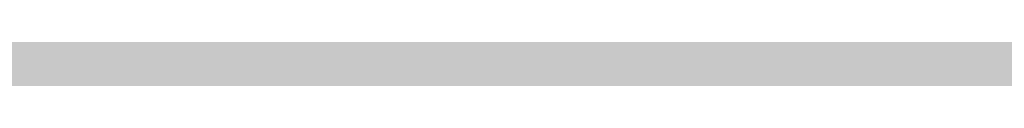
# Model space of a CAD drawing. Units: millimetres. Extents: x 0 to 2267, y 0 to 1823.
# Tile 172 of 256: x 1833.606 to 1838.83, y 1127.431 to 1127.583. Entities that reach past the tile are written whole.
import ezdxf

# ---------------------------------------------------------------- set-up
doc = ezdxf.new("R2010")
doc.units = ezdxf.units.MM
doc.header["$MEASUREMENT"] = 0
doc.layers.add('M-HATC', color=252, linetype='Continuous', lineweight=18)

msp = doc.modelspace()

# ---------------------------------------------------------------- hatches: boundary and pattern name
at = {"layer": 'M-HATC'}
h = msp.add_hatch(color=256, dxfattribs=at)
h.dxf.hatch_style = 1
h.paths.add_polyline_path([(2055.771, 1603.062), (1381.0868, 1603.062), (1381.0868, 1598.062), (2055.771, 1598.062)])
h.paths.add_polyline_path([(2055.771, 1598.062), (1381.0868, 1598.062), (1381.0868, 1593.062), (2055.771, 1593.062)])
h.paths.add_polyline_path([(2051.3074, 1536.7609), (1385.5504, 1536.7609), (1385.5504, 1526.7609), (1387.5504, 1526.7609), (1388.5366, 1525.0528), (1385.3319, 1521.2335), (1385.3319, 1521.2226), (2050.2542, 1522.7491), (2048.3212, 1525.0528), (2049.3074, 1526.7609), (2051.3074, 1526.7609)])
edge = h.paths.add_edge_path()
edge.add_arc((1847.5345, 1379.1492), 135, 222.603061, 222.890851, ccw=False)
edge.add_line((1748.1663, 1287.7656), (1683.0921, 1287.7656))
edge.add_arc((1583.7239, 1379.1492), 135, 317.109149, 317.396939, ccw=False)
edge.add_arc((1678.9686, 1290.6707), 5, 222.8909, 317.1091, ccw=False)
edge.add_arc((1774.2133, 1379.1492), 135, 222.603061, 222.890851, ccw=False)
edge.add_line((1674.8451, 1287.7656), (1609.7709, 1287.7656))
edge.add_arc((1510.4027, 1379.1492), 135, 317.109149, 317.396939, ccw=False)
edge.add_arc((1605.6474, 1290.6707), 5, 222.8909, 317.1091, ccw=False)
edge.add_arc((1700.8921, 1379.1492), 135, 222.603061, 222.890851, ccw=False)
edge.add_line((1601.5239, 1287.7656), (1536.4497, 1287.7656))
edge.add_arc((1437.0815, 1379.1492), 135, 317.109149, 317.396939, ccw=False)
edge.add_arc((1532.3262, 1290.6707), 5, 222.8909, 317.1091, ccw=False)
edge.add_arc((1627.5709, 1379.1492), 135, 222.603061, 222.890851, ccw=False)
edge.add_line((1528.2027, 1287.7656), (1505.9289, 1287.7656))
edge.add_spline(control_points=[(1505.9289, 1287.7656), (1504.2622, 1287.7656), (1504.2622, 1282.7656), (1505.9289, 1282.7656)], knot_values=[0, 0, 0, 0, 5, 5, 5, 5], degree=3, periodic=0)
edge.add_line((1505.9289, 1282.7656), (1930.9289, 1282.7656))
edge.add_spline(control_points=[(1930.9289, 1282.7656), (1932.5956, 1282.7656), (1932.5956, 1287.7656), (1930.9289, 1287.7656)], knot_values=[0, 0, 0, 0, 5, 5, 5, 5], degree=3, periodic=0)
edge.add_line((1930.9289, 1287.7656), (1903.0557, 1287.7656))
edge.add_arc((1803.6875, 1379.1492), 135, 317.109149, 317.396939, ccw=False)
edge.add_arc((1898.9322, 1290.6707), 5, 222.8909, 317.1091, ccw=False)
edge.add_arc((1994.1769, 1379.1492), 135, 222.603061, 222.890851, ccw=False)
edge.add_line((1894.8087, 1287.7656), (1829.7345, 1287.7656))
edge.add_arc((1730.3663, 1379.1492), 135, 317.109149, 317.396939, ccw=False)
edge.add_arc((1825.611, 1290.6707), 5, 222.8909, 317.1091, ccw=False)
edge.add_arc((1920.8557, 1379.1492), 135, 222.603061, 222.890851, ccw=False)
edge.add_line((1821.4875, 1287.7656), (1756.4133, 1287.7656))
edge.add_arc((1657.0451, 1379.1492), 135, 317.109149, 317.396939, ccw=False)
edge.add_arc((1752.2898, 1290.6707), 5, 222.8909, 317.1091, ccw=False)
edge = h.paths.add_edge_path()
edge.add_spline(control_points=[(1843.4289, 1227.2475), (1845.0956, 1227.2475), (1845.0956, 1232.2475), (1843.4289, 1232.2475)], knot_values=[0, 0, 0, 0, 5, 5, 5, 5], degree=3, periodic=0)
edge.add_line((1843.4289, 1232.2475), (1593.4289, 1232.2475))
edge.add_spline(control_points=[(1593.4289, 1232.2475), (1591.7622, 1232.2475), (1591.7622, 1227.2475), (1593.4289, 1227.2475)], knot_values=[0, 0, 0, 0, 5, 5, 5, 5], degree=3, periodic=0)
edge.add_line((1593.4289, 1227.2475), (1843.4289, 1227.2475))
h.paths.add_polyline_path([(1905.9289, 1127.4171), (1530.9289, 1127.4171, 0.414214), (1520.9289, 1117.4171), (1530.9289, 1117.4171), (1915.9289, 1117.4171, 0.414214)])
edge = h.paths.add_edge_path()
edge.add_arc((1397.0858, 1498.4078), 12.7299, 90.78215, 190.87871, ccw=False)
edge.add_line((1396.912, 1511.1365), (1428.0097, 1511.3488))
edge.add_line((1428.0097, 1511.3488), (1433.0097, 1511.3488))
edge.add_line((1433.0097, 1511.3488), (1434.439, 1511.3488))
edge.add_arc((1419.474, 1498.0804), 20, 41.561, 74.08211)
edge.add_line((1424.9592, 1517.3135), (1399.9351, 1517.2561))
edge.add_spline(control_points=[(1399.9307, 1517.2561), (1399.884, 1517.2131), (1399.8328, 1517.1689), (1399.7774, 1517.1236)], knot_values=[11.567499, 11.567499, 11.567499, 11.567499, 11.814249, 11.814249, 11.814249, 11.814249], degree=3, periodic=0)
edge.add_spline(control_points=[(1399.6328, 1517.0099), (1399.5831, 1516.9721), (1399.5307, 1516.9338), (1399.4759, 1516.8947)], knot_values=[11.167718, 11.167718, 11.167718, 11.167718, 11.365188, 11.365188, 11.365188, 11.365188], degree=3, periodic=0)
edge.add_spline(control_points=[(1399.3398, 1516.8001), (1399.1514, 1516.6719), (1398.9384, 1516.5377), (1398.704, 1516.3994)], knot_values=[10.376405, 10.376405, 10.376405, 10.376405, 11.00994, 11.00994, 11.00994, 11.00994], degree=3, periodic=0)
edge.add_spline(control_points=[(1398.6572, 1516.3719), (1398.5789, 1516.326), (1398.4983, 1516.2797), (1398.4155, 1516.2331)], knot_values=[10.125175, 10.125175, 10.125175, 10.125175, 10.334406, 10.334406, 10.334406, 10.334406], degree=3, periodic=0)
edge.add_spline(control_points=[(1398.2642, 1516.1487), (1398.196, 1516.1111), (1398.1263, 1516.0732), (1398.0555, 1516.0351)], knot_values=[9.832246, 9.832246, 9.832246, 9.832246, 9.999658, 9.999658, 9.999658, 9.999658], degree=3, periodic=0)
edge.add_spline(control_points=[(1397.9987, 1516.0048), (1397.7312, 1515.8621), (1397.446, 1515.7171), (1397.1466, 1515.5714)], knot_values=[9.161808, 9.161808, 9.161808, 9.161808, 9.787769, 9.787769, 9.787769, 9.787769], degree=3, periodic=0)
edge.add_spline(control_points=[(1397.1466, 1515.5714), (1396.8418, 1515.423), (1396.5222, 1515.274), (1396.1914, 1515.1262)], knot_values=[8.524455, 8.524455, 8.524455, 8.524455, 9.161808, 9.161808, 9.161808, 9.161808], degree=3, periodic=0)
edge.add_spline(control_points=[(1396.0777, 1515.0756), (1395.9854, 1515.0348), (1395.8922, 1514.994), (1395.7983, 1514.9534)], knot_values=[8.275193, 8.275193, 8.275193, 8.275193, 8.451726, 8.451726, 8.451726, 8.451726], degree=3, periodic=0)
edge.add_spline(control_points=[(1395.6018, 1514.8691), (1395.4997, 1514.8257), (1395.3968, 1514.7824), (1395.2932, 1514.7394)], knot_values=[7.962917, 7.962917, 7.962917, 7.962917, 8.152764, 8.152764, 8.152764, 8.152764], degree=3, periodic=0)
edge.add_spline(control_points=[(1395.2116, 1514.7057), (1394.8278, 1514.5475), (1394.4345, 1514.3929), (1394.0364, 1514.2442)], knot_values=[7.21254, 7.21254, 7.21254, 7.21254, 7.913148, 7.913148, 7.913148, 7.913148], degree=3, periodic=0)
edge.add_spline(control_points=[(1394.0364, 1514.2442), (1393.7076, 1514.1214), (1393.3754, 1514.0027), (1393.0427, 1513.8895)], knot_values=[6.633733, 6.633733, 6.633733, 6.633733, 7.21254, 7.21254, 7.21254, 7.21254], degree=3, periodic=0)
edge.add_spline(control_points=[(1392.8214, 1513.815), (1392.7198, 1513.7812), (1392.6181, 1513.7479), (1392.5166, 1513.7152)], knot_values=[6.328796, 6.328796, 6.328796, 6.328796, 6.505493, 6.505493, 6.505493, 6.505493], degree=3, periodic=0)
edge.add_spline(control_points=[(1392.5166, 1513.7152), (1392.3187, 1513.6515), (1392.1212, 1513.59), (1391.9244, 1513.531)], knot_values=[5.984605, 5.984605, 5.984605, 5.984605, 6.328796, 6.328796, 6.328796, 6.328796], degree=3, periodic=0)
edge.add_spline(control_points=[(1391.7915, 1513.4915), (1391.3122, 1513.3501), (1390.8384, 1513.2239), (1390.3784, 1513.1171)], knot_values=[5.066697, 5.066697, 5.066697, 5.066697, 5.907055, 5.907055, 5.907055, 5.907055], degree=3, periodic=0)
edge.add_spline(control_points=[(1390.3784, 1513.1171), (1390.1797, 1513.071), (1389.9836, 1513.0284), (1389.7907, 1512.9899)], knot_values=[4.70367, 4.70367, 4.70367, 4.70367, 5.066695, 5.066695, 5.066695, 5.066695], degree=3, periodic=0)
edge.add_spline(control_points=[(1389.422, 1512.9204), (1389.2459, 1512.8892), (1389.0729, 1512.8617), (1388.9036, 1512.8381)], knot_values=[4.130571, 4.130571, 4.130571, 4.130571, 4.469816, 4.469816, 4.469816, 4.469816], degree=3, periodic=0)
edge.add_spline(control_points=[(1388.9036, 1512.8381), (1388.591, 1512.7946), (1388.2911, 1512.7644), (1388.0071, 1512.7494)], knot_values=[3.504031, 3.504031, 3.504031, 3.504031, 4.130571, 4.130571, 4.130571, 4.130571], degree=3, periodic=0)
edge.add_spline(control_points=[(1387.9356, 1512.7459), (1387.8538, 1512.7423), (1387.7733, 1512.74), (1387.6944, 1512.739)], knot_values=[3.268866, 3.268866, 3.268866, 3.268866, 3.451164, 3.451164, 3.451164, 3.451164], degree=3, periodic=0)
edge.add_spline(control_points=[(1387.3351, 1512.7443), (1387.2076, 1512.7499), (1387.0847, 1512.7597), (1386.967, 1512.7739)], knot_values=[2.670686, 2.670686, 2.670686, 2.670686, 2.984, 2.984, 2.984, 2.984], degree=3, periodic=0)
edge.add_spline(control_points=[(1386.8327, 1512.7922), (1386.8209, 1512.7941), (1386.8092, 1512.7959), (1386.7975, 1512.7979)], knot_values=[2.516981, 2.516981, 2.516981, 2.516981, 2.549528, 2.549528, 2.549528, 2.549528], degree=3, periodic=0)
edge.add_spline(control_points=[(1386.4526, 1512.8735), (1386.4257, 1512.881), (1386.3993, 1512.889), (1386.3733, 1512.8972)], knot_values=[2.095869, 2.095869, 2.095869, 2.095869, 2.17941, 2.17941, 2.17941, 2.17941], degree=3, periodic=0)
edge.add_spline(control_points=[(1386.0691, 1513.0189), (1386.0634, 1513.0217), (1386.0577, 1513.0246), (1386.052, 1513.0275)], knot_values=[1.72453, 1.72453, 1.72453, 1.72453, 1.745933, 1.745933, 1.745933, 1.745933], degree=3, periodic=0)
edge.add_arc((1399.474, 1498.0804), 20, 131.82432, 180)
edge.add_arc((1630.3336, 1505.5484), 250.9708, 181.705176, 236.427975)
edge.add_arc((1605.3399, 1483.3044), 218.7822, 238.660829, 243.34961)
edge.add_arc((1647.0911, 1510.3592), 262.8986, 183.129836, 237.853442, ccw=False)
h.paths.add_polyline_path([(1406.5369, 1391.9644, 0.149382), (1491.5506, 1296.4418, -0.129517)], flags=17)
edge = h.paths.add_edge_path()
edge.add_arc((2037.3838, 1498.0804), 20, 0, 48.26587)
edge.add_spline(control_points=[(2050.6973, 1513.0052), (2050.6512, 1512.9847), (2050.6034, 1512.9655), (2050.5539, 1512.9477)], knot_values=[1.835652, 1.835652, 1.835652, 1.835652, 2.000781, 2.000781, 2.000781, 2.000781], degree=3, periodic=0)
edge.add_spline(control_points=[(2050.4616, 1512.9166), (2050.479, 1512.9221), (2050.4963, 1512.9277), (2050.5133, 1512.9335)], knot_values=[2.045477, 2.045477, 2.045477, 2.045477, 2.101389, 2.101389, 2.101389, 2.101389], degree=3, periodic=0)
edge.add_spline(control_points=[(2050.129, 1512.8342), (2050.1984, 1512.8473), (2050.2657, 1512.8623), (2050.3308, 1512.8792)], knot_values=[2.237629, 2.237629, 2.237629, 2.237629, 2.435841, 2.435841, 2.435841, 2.435841], degree=3, periodic=0)
edge.add_spline(control_points=[(2050.0946, 1512.8278), (2050.1061, 1512.8299), (2050.1176, 1512.832), (2050.129, 1512.8342)], knot_values=[2.435841, 2.435841, 2.435841, 2.435841, 2.468321, 2.468321, 2.468321, 2.468321], degree=3, periodic=0)
edge.add_spline(control_points=[(2049.7843, 1512.7851), (2049.8552, 1512.7922), (2049.9243, 1512.8008), (2049.9917, 1512.8109)], knot_values=[2.563852, 2.563852, 2.563852, 2.563852, 2.748541, 2.748541, 2.748541, 2.748541], degree=3, periodic=0)
edge.add_spline(control_points=[(2049.4052, 1512.7617), (2049.5364, 1512.7653), (2049.6629, 1512.773), (2049.7843, 1512.7851)], knot_values=[2.748541, 2.748541, 2.748541, 2.748541, 3.064882, 3.064882, 3.064882, 3.064882], degree=3, periodic=0)
edge.add_spline(control_points=[(2049.1698, 1512.7597), (2049.2336, 1512.7591), (2049.2965, 1512.7594), (2049.3584, 1512.7606)], knot_values=[3.102309, 3.102309, 3.102309, 3.102309, 3.2503, 3.2503, 3.2503, 3.2503], degree=3, periodic=0)
edge.add_spline(control_points=[(2048.8573, 1512.7691), (2048.9638, 1512.7638), (2049.068, 1512.7606), (2049.1698, 1512.7597)], knot_values=[3.2503, 3.2503, 3.2503, 3.2503, 3.486069, 3.486069, 3.486069, 3.486069], degree=3, periodic=0)
edge.add_spline(control_points=[(2048.6924, 1512.7789), (2048.3729, 1512.8009), (2048.0345, 1512.8411), (2047.6817, 1512.897)], knot_values=[3.606429, 3.606429, 3.606429, 3.606429, 4.2989, 4.2989, 4.2989, 4.2989], degree=3, periodic=0)
edge.add_spline(control_points=[(2047.6817, 1512.897), (2047.5458, 1512.9185), (2047.4077, 1512.9424), (2047.2678, 1512.9685)], knot_values=[4.2989, 4.2989, 4.2989, 4.2989, 4.565769, 4.565769, 4.565769, 4.565769], degree=3, periodic=0)
edge.add_spline(control_points=[(2047.2678, 1512.9685), (2047.1449, 1512.9914), (2047.0207, 1513.016), (2046.8951, 1513.0422)], knot_values=[4.565769, 4.565769, 4.565769, 4.565769, 4.799971, 4.799971, 4.799971, 4.799971], degree=3, periodic=0)
edge.add_spline(control_points=[(2046.8951, 1513.0422), (2046.5286, 1513.1188), (2046.1513, 1513.209), (2045.7676, 1513.3107)], knot_values=[4.799971, 4.799971, 4.799971, 4.799971, 5.483718, 5.483718, 5.483718, 5.483718], degree=3, periodic=0)
edge.add_spline(control_points=[(2045.7676, 1513.3107), (2045.3724, 1513.4154), (2044.9704, 1513.5322), (2044.5662, 1513.6588)], knot_values=[5.483718, 5.483718, 5.483718, 5.483718, 6.187866, 6.187866, 6.187866, 6.187866], degree=3, periodic=0)
edge.add_spline(control_points=[(2044.5662, 1513.6588), (2044.4149, 1513.7061), (2044.2633, 1513.7549), (2044.1116, 1513.8048)], knot_values=[6.187866, 6.187866, 6.187866, 6.187866, 6.451551, 6.451551, 6.451551, 6.451551], degree=3, periodic=0)
edge.add_spline(control_points=[(2044.1116, 1513.8048), (2043.9967, 1513.8427), (2043.8817, 1513.8813), (2043.7668, 1513.9205)], knot_values=[6.451551, 6.451551, 6.451551, 6.451551, 6.651434, 6.651434, 6.651434, 6.651434], degree=3, periodic=0)
edge.add_spline(control_points=[(2043.7668, 1513.9205), (2043.3716, 1514.0554), (2042.9774, 1514.1979), (2042.5886, 1514.3458)], knot_values=[6.651434, 6.651434, 6.651434, 6.651434, 7.338879, 7.338879, 7.338879, 7.338879], degree=3, periodic=0)
edge.add_spline(control_points=[(2042.5886, 1514.3458), (2042.1643, 1514.5071), (2041.7465, 1514.6749), (2041.3409, 1514.846)], knot_values=[7.338879, 7.338879, 7.338879, 7.338879, 8.089209, 8.089209, 8.089209, 8.089209], degree=3, periodic=0)
edge.add_spline(control_points=[(2041.3409, 1514.846), (2041.1028, 1514.9465), (2040.869, 1515.0481), (2040.6405, 1515.1502)], knot_values=[8.089209, 8.089209, 8.089209, 8.089209, 8.529587, 8.529587, 8.529587, 8.529587], degree=3, periodic=0)
edge.add_spline(control_points=[(2040.51, 1515.2089), (2040.0824, 1515.4022), (2039.6747, 1515.5971), (2039.295, 1515.7894)], knot_values=[8.613818, 8.613818, 8.613818, 8.613818, 9.44571, 9.44571, 9.44571, 9.44571], degree=3, periodic=0)
edge.add_spline(control_points=[(2039.295, 1515.7894), (2039.0618, 1515.9075), (2038.8391, 1516.0246), (2038.6288, 1516.1398)], knot_values=[9.44571, 9.44571, 9.44571, 9.44571, 9.956404, 9.956404, 9.956404, 9.956404], degree=3, periodic=0)
edge.add_spline(control_points=[(2038.6288, 1516.1398), (2038.5187, 1516.2001), (2038.4121, 1516.2598), (2038.309, 1516.3189)], knot_values=[9.956404, 9.956404, 9.956404, 9.956404, 10.223542, 10.223542, 10.223542, 10.223542], degree=3, periodic=0)
edge.add_spline(control_points=[(2038.309, 1516.3189), (2038.2138, 1516.3735), (2038.1216, 1516.4276), (2038.0328, 1516.481)], knot_values=[10.223542, 10.223542, 10.223542, 10.223542, 10.47051, 10.47051, 10.47051, 10.47051], degree=3, periodic=0)
edge.add_spline(control_points=[(2038.0328, 1516.481), (2037.7855, 1516.6296), (2037.5639, 1516.773), (2037.3722, 1516.909)], knot_values=[10.47051, 10.47051, 10.47051, 10.47051, 11.15767, 11.15767, 11.15767, 11.15767], degree=3, periodic=0)
edge.add_spline(control_points=[(2037.3722, 1516.909), (2037.2789, 1516.9752), (2037.1927, 1517.0396), (2037.1142, 1517.102)], knot_values=[11.15767, 11.15767, 11.15767, 11.15767, 11.49227, 11.49227, 11.49227, 11.49227], degree=3, periodic=0)
edge.add_spline(control_points=[(2036.8564, 1517.3259), (2036.9148, 1517.2692), (2036.9814, 1517.2103), (2037.0557, 1517.1492)], knot_values=[11.577341, 11.577341, 11.577341, 11.577341, 11.91035, 11.91035, 11.91035, 11.91035], degree=3, periodic=0)
edge.add_spline(control_points=[(2036.8074, 1517.3748), (2036.823, 1517.3587), (2036.8393, 1517.3424), (2036.8564, 1517.3259)], knot_values=[11.91035, 11.91035, 11.91035, 11.91035, 12.007402, 12.007402, 12.007402, 12.007402], degree=3, periodic=0)
edge.add_spline(control_points=[(2036.7017, 1517.494), (2036.7104, 1517.483), (2036.7196, 1517.4719), (2036.7291, 1517.4606)], knot_values=[12.184155, 12.184155, 12.184155, 12.184155, 12.255409, 12.255409, 12.255409, 12.255409], degree=3, periodic=0)
edge.add_spline(control_points=[(2036.6159, 1517.6205), (2036.62, 1517.613), (2036.6243, 1517.6055), (2036.6289, 1517.5979)], knot_values=[12.487913, 12.487913, 12.487913, 12.487913, 12.541035, 12.541035, 12.541035, 12.541035], degree=3, periodic=0)
edge.add_spline(control_points=[(2036.5635, 1517.786), (2036.5637, 1517.7794), (2036.5642, 1517.7726), (2036.565, 1517.7658)], knot_values=[12.911761, 12.911761, 12.911761, 12.911761, 12.968286, 12.968286, 12.968286, 12.968286], degree=3, periodic=0)
edge.add_spline(control_points=[(2036.6166, 1517.9304), (2036.6125, 1517.9259), (2036.6086, 1517.9212), (2036.6049, 1517.9165)], knot_values=[13.382527, 13.382527, 13.382527, 13.382527, 13.433791, 13.433791, 13.433791, 13.433791], degree=3, periodic=0)
edge.add_spline(control_points=[(2036.749, 1518.017), (2036.7361, 1518.0116), (2036.7239, 1518.006), (2036.7124, 1518.0002)], knot_values=[13.726299, 13.726299, 13.726299, 13.726299, 13.809928, 13.809928, 13.809928, 13.809928], degree=3, periodic=0)
edge.add_spline(control_points=[(2036.8604, 1518.0528), (2036.8386, 1518.0474), (2036.8181, 1518.0416), (2036.7988, 1518.0353)], knot_values=[13.910887, 13.910887, 13.910887, 13.910887, 14.02153, 14.02153, 14.02153, 14.02153], degree=3, periodic=0)
edge.add_line((2036.9639, 1518.0804), (2032.3838, 1518.0804))
edge.add_line((2032.3838, 1518.0804), (2027.3838, 1518.0804))
edge.add_line((2027.3838, 1518.0804), (2022.3838, 1518.0804))
edge.add_line((2022.3838, 1518.0804), (2017.3838, 1518.0804))
edge.add_arc((2017.3838, 1498.0804), 20, 90, 138.439)
edge.add_line((2002.4188, 1511.3488), (2003.8481, 1511.3488))
edge.add_line((2003.8481, 1511.3488), (2008.8481, 1511.3488))
edge.add_line((2008.8481, 1511.3488), (2039.772, 1511.1377))
edge.add_arc((2039.772, 1498.4078), 12.7299, -10.87871, 90, ccw=False)
edge.add_arc((1789.7668, 1510.3592), 262.8986, 302.146558, 356.870164, ccw=False)
edge.add_arc((1831.5179, 1483.3044), 218.7822, 296.65039, 301.339171)
edge.add_arc((1806.5242, 1505.5484), 250.9708, 303.572025, 358.294824)
h.paths.add_polyline_path([(2030.321, 1391.9644, -0.129517), (1945.3072, 1296.4418, 0.149382)], flags=17)
edge = h.paths.add_edge_path()
edge.add_spline(control_points=[(2037.2464, 1518.0821), (2037.2898, 1518.081), (2037.3355, 1518.0804), (2037.3838, 1518.0804)], knot_values=[0.000012, 0.000012, 0.000012, 0.000012, 0.144754, 0.144754, 0.144754, 0.144754], degree=3, periodic=0)
edge.add_line((2037.3357, 1518.0804), (2037.0096, 1518.0804))
edge.add_spline(control_points=[(2037.0096, 1518.0804), (2036.9822, 1518.0768), (2036.956, 1518.0727), (2036.9312, 1518.0681)], knot_values=[14.13465, 14.13465, 14.13465, 14.13465, 14.247197, 14.247197, 14.247197, 14.247197], degree=3, periodic=0)
edge.add_spline(control_points=[(2036.9312, 1518.0681), (2036.9276, 1518.0674), (2036.9241, 1518.0667), (2036.9205, 1518.0661)], knot_values=[14.118315, 14.118315, 14.118315, 14.118315, 14.13465, 14.13465, 14.13465, 14.13465], degree=3, periodic=0)
edge.add_spline(control_points=[(2036.9205, 1518.0661), (2036.9118, 1518.0644), (2036.9032, 1518.0626), (2036.8948, 1518.0608)], knot_values=[14.078086, 14.078086, 14.078086, 14.078086, 14.118315, 14.118315, 14.118315, 14.118315], degree=3, periodic=0)
edge.add_spline(control_points=[(2036.8948, 1518.0608), (2036.883, 1518.0583), (2036.8716, 1518.0556), (2036.8604, 1518.0528)], knot_values=[14.02153, 14.02153, 14.02153, 14.02153, 14.078086, 14.078086, 14.078086, 14.078086], degree=3, periodic=0)
edge.add_spline(control_points=[(2036.8604, 1518.0528), (2036.8386, 1518.0474), (2036.8181, 1518.0416), (2036.7988, 1518.0353)], knot_values=[13.910887, 13.910887, 13.910887, 13.910887, 14.02153, 14.02153, 14.02153, 14.02153], degree=3, periodic=0)
edge.add_spline(control_points=[(2036.7988, 1518.0353), (2036.7981, 1518.035), (2036.7974, 1518.0348), (2036.7967, 1518.0346)], knot_values=[13.906906, 13.906906, 13.906906, 13.906906, 13.910887, 13.910887, 13.910887, 13.910887], degree=3, periodic=0)
edge.add_spline(control_points=[(2036.7967, 1518.0346), (2036.7882, 1518.0318), (2036.7799, 1518.0289), (2036.7719, 1518.0259)], knot_values=[13.857826, 13.857826, 13.857826, 13.857826, 13.906906, 13.906906, 13.906906, 13.906906], degree=3, periodic=0)
edge.add_spline(control_points=[(2036.7719, 1518.0259), (2036.764, 1518.023), (2036.7564, 1518.02), (2036.749, 1518.017)], knot_values=[13.809928, 13.809928, 13.809928, 13.809928, 13.857826, 13.857826, 13.857826, 13.857826], degree=3, periodic=0)
edge.add_spline(control_points=[(2036.749, 1518.017), (2036.7361, 1518.0116), (2036.7239, 1518.006), (2036.7124, 1518.0002)], knot_values=[13.726299, 13.726299, 13.726299, 13.726299, 13.809928, 13.809928, 13.809928, 13.809928], degree=3, periodic=0)
edge.add_spline(control_points=[(2036.7124, 1518.0002), (2036.7121, 1518), (2036.7118, 1517.9999), (2036.7115, 1517.9997)], knot_values=[13.723993, 13.723993, 13.723993, 13.723993, 13.726299, 13.726299, 13.726299, 13.726299], degree=3, periodic=0)
edge.add_spline(control_points=[(2036.7115, 1517.9997), (2036.7063, 1517.9971), (2036.7013, 1517.9944), (2036.6965, 1517.9917)], knot_values=[13.686536, 13.686536, 13.686536, 13.686536, 13.723993, 13.723993, 13.723993, 13.723993], degree=3, periodic=0)
edge.add_spline(control_points=[(2036.6965, 1517.9917), (2036.6919, 1517.9891), (2036.6874, 1517.9865), (2036.6831, 1517.9839)], knot_values=[13.651251, 13.651251, 13.651251, 13.651251, 13.686536, 13.686536, 13.686536, 13.686536], degree=3, periodic=0)
edge.add_spline(control_points=[(2036.6831, 1517.9839), (2036.6764, 1517.9798), (2036.67, 1517.9757), (2036.6639, 1517.9714)], knot_values=[13.596804, 13.596804, 13.596804, 13.596804, 13.651251, 13.651251, 13.651251, 13.651251], degree=3, periodic=0)
edge.add_spline(control_points=[(2036.6639, 1517.9714), (2036.6636, 1517.9712), (2036.6633, 1517.9709), (2036.6629, 1517.9707)], knot_values=[13.593956, 13.593956, 13.593956, 13.593956, 13.596804, 13.596804, 13.596804, 13.596804], degree=3, periodic=0)
edge.add_spline(control_points=[(2036.6629, 1517.9707), (2036.6603, 1517.9689), (2036.6577, 1517.967), (2036.6552, 1517.9651)], knot_values=[13.570322, 13.570322, 13.570322, 13.570322, 13.593956, 13.593956, 13.593956, 13.593956], degree=3, periodic=0)
edge.add_spline(control_points=[(2036.6552, 1517.9651), (2036.6525, 1517.9631), (2036.6499, 1517.9611), (2036.6474, 1517.9591)], knot_values=[13.545477, 13.545477, 13.545477, 13.545477, 13.570322, 13.570322, 13.570322, 13.570322], degree=3, periodic=0)
edge.add_spline(control_points=[(2036.6474, 1517.9591), (2036.6472, 1517.9589), (2036.6471, 1517.9588), (2036.6469, 1517.9587)], knot_values=[13.543931, 13.543931, 13.543931, 13.543931, 13.545477, 13.545477, 13.545477, 13.545477], degree=3, periodic=0)
edge.add_spline(control_points=[(2036.6469, 1517.9587), (2036.6412, 1517.9541), (2036.6358, 1517.9494), (2036.6307, 1517.9447)], knot_values=[13.488237, 13.488237, 13.488237, 13.488237, 13.543931, 13.543931, 13.543931, 13.543931], degree=3, periodic=0)
edge.add_spline(control_points=[(2036.6307, 1517.9447), (2036.6282, 1517.9423), (2036.6257, 1517.9399), (2036.6233, 1517.9374)], knot_values=[13.460307, 13.460307, 13.460307, 13.460307, 13.488237, 13.488237, 13.488237, 13.488237], degree=3, periodic=0)
edge.add_spline(control_points=[(2036.6233, 1517.9374), (2036.6215, 1517.9356), (2036.6198, 1517.9338), (2036.6181, 1517.932)], knot_values=[13.439712, 13.439712, 13.439712, 13.439712, 13.460307, 13.460307, 13.460307, 13.460307], degree=3, periodic=0)
edge.add_spline(control_points=[(2036.6181, 1517.932), (2036.6176, 1517.9315), (2036.6171, 1517.9309), (2036.6166, 1517.9304)], knot_values=[13.433791, 13.433791, 13.433791, 13.433791, 13.439712, 13.439712, 13.439712, 13.439712], degree=3, periodic=0)
edge.add_spline(control_points=[(2036.6166, 1517.9304), (2036.6125, 1517.9259), (2036.6086, 1517.9212), (2036.6049, 1517.9165)], knot_values=[13.382527, 13.382527, 13.382527, 13.382527, 13.433791, 13.433791, 13.433791, 13.433791], degree=3, periodic=0)
edge.add_spline(control_points=[(2036.6049, 1517.9165), (2036.6026, 1517.9135), (2036.6004, 1517.9104), (2036.5982, 1517.9074)], knot_values=[13.350017, 13.350017, 13.350017, 13.350017, 13.382527, 13.382527, 13.382527, 13.382527], degree=3, periodic=0)
edge.add_spline(control_points=[(2036.5982, 1517.9074), (2036.5972, 1517.9059), (2036.5962, 1517.9043), (2036.5952, 1517.9028)], knot_values=[13.333922, 13.333922, 13.333922, 13.333922, 13.350017, 13.350017, 13.350017, 13.350017], degree=3, periodic=0)
edge.add_spline(control_points=[(2036.5952, 1517.9028), (2036.5945, 1517.9018), (2036.5939, 1517.9009), (2036.5933, 1517.8999)], knot_values=[13.323828, 13.323828, 13.323828, 13.323828, 13.333922, 13.333922, 13.333922, 13.333922], degree=3, periodic=0)
edge.add_spline(control_points=[(2036.5933, 1517.8999), (2036.5905, 1517.8955), (2036.5879, 1517.8909), (2036.5855, 1517.8864)], knot_values=[13.277545, 13.277545, 13.277545, 13.277545, 13.323828, 13.323828, 13.323828, 13.323828], degree=3, periodic=0)
edge.add_spline(control_points=[(2036.5855, 1517.8864), (2036.5836, 1517.8827), (2036.5817, 1517.8789), (2036.5801, 1517.8751)], knot_values=[13.240119, 13.240119, 13.240119, 13.240119, 13.277545, 13.277545, 13.277545, 13.277545], degree=3, periodic=0)
edge.add_spline(control_points=[(2036.5801, 1517.8751), (2036.5795, 1517.8739), (2036.579, 1517.8727), (2036.5785, 1517.8715)], knot_values=[13.228211, 13.228211, 13.228211, 13.228211, 13.240119, 13.240119, 13.240119, 13.240119], degree=3, periodic=0)
edge.add_spline(control_points=[(2036.5785, 1517.8715), (2036.578, 1517.8702), (2036.5774, 1517.869), (2036.5769, 1517.8677)], knot_values=[13.215717, 13.215717, 13.215717, 13.215717, 13.228211, 13.228211, 13.228211, 13.228211], degree=3, periodic=0)
edge.add_spline(control_points=[(2036.5769, 1517.8677), (2036.5755, 1517.864), (2036.5741, 1517.8603), (2036.5729, 1517.8565)], knot_values=[13.179847, 13.179847, 13.179847, 13.179847, 13.215717, 13.215717, 13.215717, 13.215717], degree=3, periodic=0)
edge.add_spline(control_points=[(2036.5729, 1517.8565), (2036.5713, 1517.8515), (2036.5699, 1517.8464), (2036.5687, 1517.8413)], knot_values=[13.132017, 13.132017, 13.132017, 13.132017, 13.179847, 13.179847, 13.179847, 13.179847], degree=3, periodic=0)
edge.add_spline(control_points=[(2036.5687, 1517.8413), (2036.5684, 1517.8402), (2036.5682, 1517.8392), (2036.568, 1517.8382)], knot_values=[13.122482, 13.122482, 13.122482, 13.122482, 13.132017, 13.132017, 13.132017, 13.132017], degree=3, periodic=0)
edge.add_spline(control_points=[(2036.568, 1517.8382), (2036.5676, 1517.8363), (2036.5672, 1517.8345), (2036.5669, 1517.8327)], knot_values=[13.105592, 13.105592, 13.105592, 13.105592, 13.122482, 13.122482, 13.122482, 13.122482], degree=3, periodic=0)
edge.add_spline(control_points=[(2036.5669, 1517.8327), (2036.5662, 1517.8292), (2036.5657, 1517.8257), (2036.5652, 1517.8222)], knot_values=[13.074063, 13.074063, 13.074063, 13.074063, 13.105592, 13.105592, 13.105592, 13.105592], degree=3, periodic=0)
edge.add_spline(control_points=[(2036.5652, 1517.8222), (2036.5652, 1517.8222), (2036.5652, 1517.8222), (2036.5652, 1517.8222)], knot_values=[13.074043, 13.074043, 13.074043, 13.074043, 13.074063, 13.074063, 13.074063, 13.074063], degree=3, periodic=0)
edge.add_spline(control_points=[(2036.5652, 1517.8222), (2036.5644, 1517.8164), (2036.5639, 1517.8106), (2036.5636, 1517.8046)], knot_values=[13.021884, 13.021884, 13.021884, 13.021884, 13.074043, 13.074043, 13.074043, 13.074043], degree=3, periodic=0)
edge.add_spline(control_points=[(2036.5636, 1517.8046), (2036.5636, 1517.804), (2036.5636, 1517.8034), (2036.5635, 1517.8028)], knot_values=[13.01674, 13.01674, 13.01674, 13.01674, 13.021884, 13.021884, 13.021884, 13.021884], degree=3, periodic=0)
edge.add_spline(control_points=[(2036.5635, 1517.8028), (2036.5634, 1517.8005), (2036.5634, 1517.7982), (2036.5634, 1517.7958)], knot_values=[12.996438, 12.996438, 12.996438, 12.996438, 13.01674, 13.01674, 13.01674, 13.01674], degree=3, periodic=0)
edge.add_spline(control_points=[(2036.5634, 1517.7958), (2036.5633, 1517.7926), (2036.5634, 1517.7893), (2036.5635, 1517.786)], knot_values=[12.968286, 12.968286, 12.968286, 12.968286, 12.996438, 12.996438, 12.996438, 12.996438], degree=3, periodic=0)
edge.add_spline(control_points=[(2036.5635, 1517.786), (2036.5637, 1517.7794), (2036.5642, 1517.7726), (2036.565, 1517.7658)], knot_values=[12.911761, 12.911761, 12.911761, 12.911761, 12.968286, 12.968286, 12.968286, 12.968286], degree=3, periodic=0)
edge.add_spline(control_points=[(2036.565, 1517.7658), (2036.565, 1517.7657), (2036.565, 1517.7656), (2036.565, 1517.7656)], knot_values=[12.911017, 12.911017, 12.911017, 12.911017, 12.911761, 12.911761, 12.911761, 12.911761], degree=3, periodic=0)
edge.add_spline(control_points=[(2036.565, 1517.7656), (2036.5654, 1517.7625), (2036.5658, 1517.7593), (2036.5663, 1517.7562)], knot_values=[12.88528, 12.88528, 12.88528, 12.88528, 12.911017, 12.911017, 12.911017, 12.911017], degree=3, periodic=0)
edge.add_spline(control_points=[(2036.5663, 1517.7562), (2036.5667, 1517.7534), (2036.5672, 1517.7506), (2036.5677, 1517.7478)], knot_values=[12.862519, 12.862519, 12.862519, 12.862519, 12.88528, 12.88528, 12.88528, 12.88528], degree=3, periodic=0)
edge.add_spline(control_points=[(2036.5677, 1517.7478), (2036.5678, 1517.7474), (2036.5679, 1517.7469), (2036.568, 1517.7465)], knot_values=[12.858885, 12.858885, 12.858885, 12.858885, 12.862519, 12.862519, 12.862519, 12.862519], degree=3, periodic=0)
edge.add_spline(control_points=[(2036.568, 1517.7465), (2036.5692, 1517.7399), (2036.5707, 1517.7332), (2036.5724, 1517.7264)], knot_values=[12.8053, 12.8053, 12.8053, 12.8053, 12.858885, 12.858885, 12.858885, 12.858885], degree=3, periodic=0)
edge.add_spline(control_points=[(2036.5724, 1517.7264), (2036.5734, 1517.7226), (2036.5745, 1517.7187), (2036.5756, 1517.7149)], knot_values=[12.775176, 12.775176, 12.775176, 12.775176, 12.8053, 12.8053, 12.8053, 12.8053], degree=3, periodic=0)
edge.add_spline(control_points=[(2036.5756, 1517.7149), (2036.5763, 1517.7125), (2036.577, 1517.7102), (2036.5778, 1517.7078)], knot_values=[12.756759, 12.756759, 12.756759, 12.756759, 12.775176, 12.775176, 12.775176, 12.775176], degree=3, periodic=0)
edge.add_spline(control_points=[(2036.5778, 1517.7078), (2036.5781, 1517.7067), (2036.5784, 1517.7057), (2036.5787, 1517.7047)], knot_values=[12.748742, 12.748742, 12.748742, 12.748742, 12.756759, 12.756759, 12.756759, 12.756759], degree=3, periodic=0)
edge.add_spline(control_points=[(2036.5787, 1517.7047), (2036.5808, 1517.6983), (2036.5831, 1517.6919), (2036.5856, 1517.6854)], knot_values=[12.69959, 12.69959, 12.69959, 12.69959, 12.748742, 12.748742, 12.748742, 12.748742], degree=3, periodic=0)
edge.add_spline(control_points=[(2036.5856, 1517.6854), (2036.5876, 1517.68), (2036.5898, 1517.6746), (2036.5921, 1517.6692)], knot_values=[12.659038, 12.659038, 12.659038, 12.659038, 12.69959, 12.69959, 12.69959, 12.69959], degree=3, periodic=0)
edge.add_spline(control_points=[(2036.5921, 1517.6692), (2036.594, 1517.6648), (2036.5959, 1517.6605), (2036.5979, 1517.6561)], knot_values=[12.626806, 12.626806, 12.626806, 12.626806, 12.659038, 12.659038, 12.659038, 12.659038], degree=3, periodic=0)
edge.add_spline(control_points=[(2036.5979, 1517.6561), (2036.5984, 1517.6551), (2036.5989, 1517.6541), (2036.5993, 1517.6531)], knot_values=[12.619394, 12.619394, 12.619394, 12.619394, 12.626806, 12.626806, 12.626806, 12.626806], degree=3, periodic=0)
edge.add_spline(control_points=[(2036.5993, 1517.6531), (2036.6043, 1517.6424), (2036.6099, 1517.6315), (2036.6159, 1517.6205)], knot_values=[12.541039, 12.541039, 12.541039, 12.541039, 12.619394, 12.619394, 12.619394, 12.619394], degree=3, periodic=0)
edge.add_spline(control_points=[(2036.6159, 1517.6205), (2036.6159, 1517.6205), (2036.6159, 1517.6205), (2036.6159, 1517.6205)], knot_values=[12.541035, 12.541035, 12.541035, 12.541035, 12.541039, 12.541039, 12.541039, 12.541039], degree=3, periodic=0)
edge.add_spline(control_points=[(2036.6159, 1517.6205), (2036.62, 1517.613), (2036.6243, 1517.6055), (2036.6289, 1517.5979)], knot_values=[12.487913, 12.487913, 12.487913, 12.487913, 12.541035, 12.541035, 12.541035, 12.541035], degree=3, periodic=0)
edge.add_spline(control_points=[(2036.6289, 1517.5979), (2036.6326, 1517.5916), (2036.6365, 1517.5853), (2036.6406, 1517.5789)], knot_values=[12.443982, 12.443982, 12.443982, 12.443982, 12.487913, 12.487913, 12.487913, 12.487913], degree=3, periodic=0)
edge.add_spline(control_points=[(2036.6406, 1517.5789), (2036.6414, 1517.5776), (2036.6423, 1517.5763), (2036.6431, 1517.5749)], knot_values=[12.434996, 12.434996, 12.434996, 12.434996, 12.443982, 12.443982, 12.443982, 12.443982], degree=3, periodic=0)
edge.add_spline(control_points=[(2036.6431, 1517.5749), (2036.6531, 1517.5596), (2036.6639, 1517.5439), (2036.6756, 1517.528)], knot_values=[12.329647, 12.329647, 12.329647, 12.329647, 12.434996, 12.434996, 12.434996, 12.434996], degree=3, periodic=0)
edge.add_spline(control_points=[(2036.6756, 1517.528), (2036.6839, 1517.5168), (2036.6925, 1517.5055), (2036.7017, 1517.494)], knot_values=[12.255409, 12.255409, 12.255409, 12.255409, 12.329647, 12.329647, 12.329647, 12.329647], degree=3, periodic=0)
edge.add_spline(control_points=[(2036.7017, 1517.494), (2036.7104, 1517.483), (2036.7196, 1517.4719), (2036.7291, 1517.4606)], knot_values=[12.184155, 12.184155, 12.184155, 12.184155, 12.255409, 12.255409, 12.255409, 12.255409], degree=3, periodic=0)
edge.add_spline(control_points=[(2036.7291, 1517.4606), (2036.7436, 1517.4435), (2036.759, 1517.4262), (2036.7753, 1517.4085)], knot_values=[12.075961, 12.075961, 12.075961, 12.075961, 12.184155, 12.184155, 12.184155, 12.184155], degree=3, periodic=0)
edge.add_spline(control_points=[(2036.7753, 1517.4085), (2036.7763, 1517.4075), (2036.7773, 1517.4064), (2036.7783, 1517.4054)], knot_values=[12.069502, 12.069502, 12.069502, 12.069502, 12.075961, 12.075961, 12.075961, 12.075961], degree=3, periodic=0)
edge.add_spline(control_points=[(2036.7783, 1517.4054), (2036.7877, 1517.3953), (2036.7974, 1517.385), (2036.8074, 1517.3748)], knot_values=[12.007402, 12.007402, 12.007402, 12.007402, 12.069502, 12.069502, 12.069502, 12.069502], degree=3, periodic=0)
edge.add_spline(control_points=[(2036.8074, 1517.3748), (2036.823, 1517.3587), (2036.8393, 1517.3424), (2036.8564, 1517.3259)], knot_values=[11.91035, 11.91035, 11.91035, 11.91035, 12.007402, 12.007402, 12.007402, 12.007402], degree=3, periodic=0)
edge.add_spline(control_points=[(2036.8564, 1517.3259), (2036.9148, 1517.2692), (2036.9814, 1517.2103), (2037.0557, 1517.1492)], knot_values=[11.577341, 11.577341, 11.577341, 11.577341, 11.91035, 11.91035, 11.91035, 11.91035], degree=3, periodic=0)
edge.add_spline(control_points=[(2037.0557, 1517.1492), (2037.0747, 1517.1336), (2037.0942, 1517.1179), (2037.1142, 1517.102)], knot_values=[11.49227, 11.49227, 11.49227, 11.49227, 11.577341, 11.577341, 11.577341, 11.577341], degree=3, periodic=0)
edge.add_spline(control_points=[(2037.1142, 1517.102), (2037.1927, 1517.0396), (2037.2789, 1516.9752), (2037.3722, 1516.909)], knot_values=[11.15767, 11.15767, 11.15767, 11.15767, 11.49227, 11.49227, 11.49227, 11.49227], degree=3, periodic=0)
edge.add_spline(control_points=[(2037.3722, 1516.909), (2037.5639, 1516.773), (2037.7855, 1516.6296), (2038.0328, 1516.481)], knot_values=[10.47051, 10.47051, 10.47051, 10.47051, 11.15767, 11.15767, 11.15767, 11.15767], degree=3, periodic=0)
edge.add_spline(control_points=[(2038.0328, 1516.481), (2038.1216, 1516.4276), (2038.2138, 1516.3735), (2038.309, 1516.3189)], knot_values=[10.223542, 10.223542, 10.223542, 10.223542, 10.47051, 10.47051, 10.47051, 10.47051], degree=3, periodic=0)
edge.add_spline(control_points=[(2038.309, 1516.3189), (2038.4121, 1516.2598), (2038.5187, 1516.2001), (2038.6288, 1516.1398)], knot_values=[9.956404, 9.956404, 9.956404, 9.956404, 10.223542, 10.223542, 10.223542, 10.223542], degree=3, periodic=0)
edge.add_spline(control_points=[(2038.6288, 1516.1398), (2038.8391, 1516.0246), (2039.0618, 1515.9075), (2039.295, 1515.7894)], knot_values=[9.44571, 9.44571, 9.44571, 9.44571, 9.956404, 9.956404, 9.956404, 9.956404], degree=3, periodic=0)
edge.add_spline(control_points=[(2039.295, 1515.7894), (2039.6747, 1515.5971), (2040.0824, 1515.4022), (2040.51, 1515.2089)], knot_values=[8.613818, 8.613818, 8.613818, 8.613818, 9.44571, 9.44571, 9.44571, 9.44571], degree=3, periodic=0)
edge.add_spline(control_points=[(2040.51, 1515.2089), (2040.5533, 1515.1893), (2040.5968, 1515.1697), (2040.6405, 1515.1502)], knot_values=[8.529587, 8.529587, 8.529587, 8.529587, 8.613818, 8.613818, 8.613818, 8.613818], degree=3, periodic=0)
edge.add_spline(control_points=[(2040.6405, 1515.1502), (2040.869, 1515.0481), (2041.1028, 1514.9465), (2041.3409, 1514.846)], knot_values=[8.089209, 8.089209, 8.089209, 8.089209, 8.529587, 8.529587, 8.529587, 8.529587], degree=3, periodic=0)
edge.add_spline(control_points=[(2041.3409, 1514.846), (2041.7465, 1514.6749), (2042.1643, 1514.5071), (2042.5886, 1514.3458)], knot_values=[7.338879, 7.338879, 7.338879, 7.338879, 8.089209, 8.089209, 8.089209, 8.089209], degree=3, periodic=0)
edge.add_spline(control_points=[(2042.5886, 1514.3458), (2042.9774, 1514.1979), (2043.3716, 1514.0554), (2043.7668, 1513.9205)], knot_values=[6.651434, 6.651434, 6.651434, 6.651434, 7.338879, 7.338879, 7.338879, 7.338879], degree=3, periodic=0)
edge.add_spline(control_points=[(2043.7668, 1513.9205), (2043.8817, 1513.8813), (2043.9967, 1513.8427), (2044.1116, 1513.8048)], knot_values=[6.451551, 6.451551, 6.451551, 6.451551, 6.651434, 6.651434, 6.651434, 6.651434], degree=3, periodic=0)
edge.add_spline(control_points=[(2044.1116, 1513.8048), (2044.2633, 1513.7549), (2044.4149, 1513.7061), (2044.5662, 1513.6588)], knot_values=[6.187866, 6.187866, 6.187866, 6.187866, 6.451551, 6.451551, 6.451551, 6.451551], degree=3, periodic=0)
edge.add_spline(control_points=[(2044.5662, 1513.6588), (2044.9704, 1513.5322), (2045.3724, 1513.4154), (2045.7676, 1513.3107)], knot_values=[5.483718, 5.483718, 5.483718, 5.483718, 6.187866, 6.187866, 6.187866, 6.187866], degree=3, periodic=0)
edge.add_spline(control_points=[(2045.7676, 1513.3107), (2046.1513, 1513.209), (2046.5286, 1513.1188), (2046.8951, 1513.0422)], knot_values=[4.799971, 4.799971, 4.799971, 4.799971, 5.483718, 5.483718, 5.483718, 5.483718], degree=3, periodic=0)
edge.add_spline(control_points=[(2046.8951, 1513.0422), (2047.0207, 1513.016), (2047.1449, 1512.9914), (2047.2678, 1512.9685)], knot_values=[4.565769, 4.565769, 4.565769, 4.565769, 4.799971, 4.799971, 4.799971, 4.799971], degree=3, periodic=0)
edge.add_spline(control_points=[(2047.2678, 1512.9685), (2047.4077, 1512.9424), (2047.5458, 1512.9185), (2047.6817, 1512.897)], knot_values=[4.2989, 4.2989, 4.2989, 4.2989, 4.565769, 4.565769, 4.565769, 4.565769], degree=3, periodic=0)
edge.add_spline(control_points=[(2047.6817, 1512.897), (2048.0345, 1512.8411), (2048.3729, 1512.8009), (2048.6924, 1512.7789)], knot_values=[3.606429, 3.606429, 3.606429, 3.606429, 4.2989, 4.2989, 4.2989, 4.2989], degree=3, periodic=0)
edge.add_spline(control_points=[(2048.6924, 1512.7789), (2048.7479, 1512.7751), (2048.8029, 1512.7718), (2048.8573, 1512.7691)], knot_values=[3.486069, 3.486069, 3.486069, 3.486069, 3.606429, 3.606429, 3.606429, 3.606429], degree=3, periodic=0)
edge.add_spline(control_points=[(2048.8573, 1512.7691), (2048.9638, 1512.7638), (2049.068, 1512.7606), (2049.1698, 1512.7597)], knot_values=[3.2503, 3.2503, 3.2503, 3.2503, 3.486069, 3.486069, 3.486069, 3.486069], degree=3, periodic=0)
edge.add_spline(control_points=[(2049.1698, 1512.7597), (2049.2336, 1512.7591), (2049.2965, 1512.7594), (2049.3584, 1512.7606)], knot_values=[3.102309, 3.102309, 3.102309, 3.102309, 3.2503, 3.2503, 3.2503, 3.2503], degree=3, periodic=0)
edge.add_spline(control_points=[(2049.3584, 1512.7606), (2049.3741, 1512.7609), (2049.3897, 1512.7613), (2049.4052, 1512.7617)], knot_values=[3.064882, 3.064882, 3.064882, 3.064882, 3.102309, 3.102309, 3.102309, 3.102309], degree=3, periodic=0)
edge.add_spline(control_points=[(2049.4052, 1512.7617), (2049.5364, 1512.7653), (2049.6629, 1512.773), (2049.7843, 1512.7851)], knot_values=[2.748541, 2.748541, 2.748541, 2.748541, 3.064882, 3.064882, 3.064882, 3.064882], degree=3, periodic=0)
edge.add_spline(control_points=[(2049.7843, 1512.7851), (2049.8552, 1512.7922), (2049.9243, 1512.8008), (2049.9917, 1512.8109)], knot_values=[2.563852, 2.563852, 2.563852, 2.563852, 2.748541, 2.748541, 2.748541, 2.748541], degree=3, periodic=0)
edge.add_spline(control_points=[(2049.9917, 1512.8109), (2050.0265, 1512.8161), (2050.0608, 1512.8218), (2050.0946, 1512.8278)], knot_values=[2.468321, 2.468321, 2.468321, 2.468321, 2.563852, 2.563852, 2.563852, 2.563852], degree=3, periodic=0)
edge.add_spline(control_points=[(2050.0946, 1512.8278), (2050.1061, 1512.8299), (2050.1176, 1512.832), (2050.129, 1512.8342)], knot_values=[2.435841, 2.435841, 2.435841, 2.435841, 2.468321, 2.468321, 2.468321, 2.468321], degree=3, periodic=0)
edge.add_spline(control_points=[(2050.129, 1512.8342), (2050.1984, 1512.8473), (2050.2657, 1512.8623), (2050.3308, 1512.8792)], knot_values=[2.237629, 2.237629, 2.237629, 2.237629, 2.435841, 2.435841, 2.435841, 2.435841], degree=3, periodic=0)
edge.add_spline(control_points=[(2050.3308, 1512.8792), (2050.3754, 1512.8908), (2050.4191, 1512.9032), (2050.4616, 1512.9166)], knot_values=[2.101389, 2.101389, 2.101389, 2.101389, 2.237629, 2.237629, 2.237629, 2.237629], degree=3, periodic=0)
edge.add_spline(control_points=[(2050.4616, 1512.9166), (2050.479, 1512.9221), (2050.4963, 1512.9277), (2050.5133, 1512.9335)], knot_values=[2.045477, 2.045477, 2.045477, 2.045477, 2.101389, 2.101389, 2.101389, 2.101389], degree=3, periodic=0)
edge.add_spline(control_points=[(2050.5133, 1512.9335), (2050.527, 1512.9382), (2050.5405, 1512.9429), (2050.5539, 1512.9477)], knot_values=[2.000781, 2.000781, 2.000781, 2.000781, 2.045477, 2.045477, 2.045477, 2.045477], degree=3, periodic=0)
edge.add_spline(control_points=[(2050.5539, 1512.9477), (2050.6034, 1512.9655), (2050.6512, 1512.9847), (2050.6973, 1513.0052)], knot_values=[1.835652, 1.835652, 1.835652, 1.835652, 2.000781, 2.000781, 2.000781, 2.000781], degree=3, periodic=0)
edge.add_arc((2037.3838, 1498.0804), 20, 48.26587, 90.12993)
edge = h.paths.add_edge_path(flags=16)
edge.add_spline(control_points=[(1386.1389, 1512.9859), (1388.92, 1511.7395), (1398.0387, 1515.5187), (1399.9307, 1517.2561)], knot_values=[1.831046, 1.831046, 1.831046, 1.831046, 11.814249, 11.814249, 11.814249, 11.814249], degree=3, periodic=0)
edge.add_line((1399.9307, 1517.2561), (1393.7435, 1517.2419))
edge.add_arc((1399.474, 1498.0804), 20, 106.6501, 131.8173)
h = msp.add_hatch(color=256, dxfattribs=at)
h.dxf.hatch_style = 1
h.paths.add_polyline_path([(2042.8886, 1580.1796), (2055.771, 1593.062), (1381.0868, 1593.062), (1393.9692, 1580.1796), (1374.086, 1560.2964), (2062.7718, 1560.2964)])
h.paths.add_polyline_path([(1843.4289, 1201.3297), (1843.4289, 1227.2475), (1593.4289, 1227.2475), (1593.4289, 1201.3297, -0.228274), (1574.5989, 1162.2346), (1530.9289, 1127.4171), (1905.9289, 1127.4171), (1862.2589, 1162.2346, -0.228274)])

doc.saveas('drawing.dxf')
